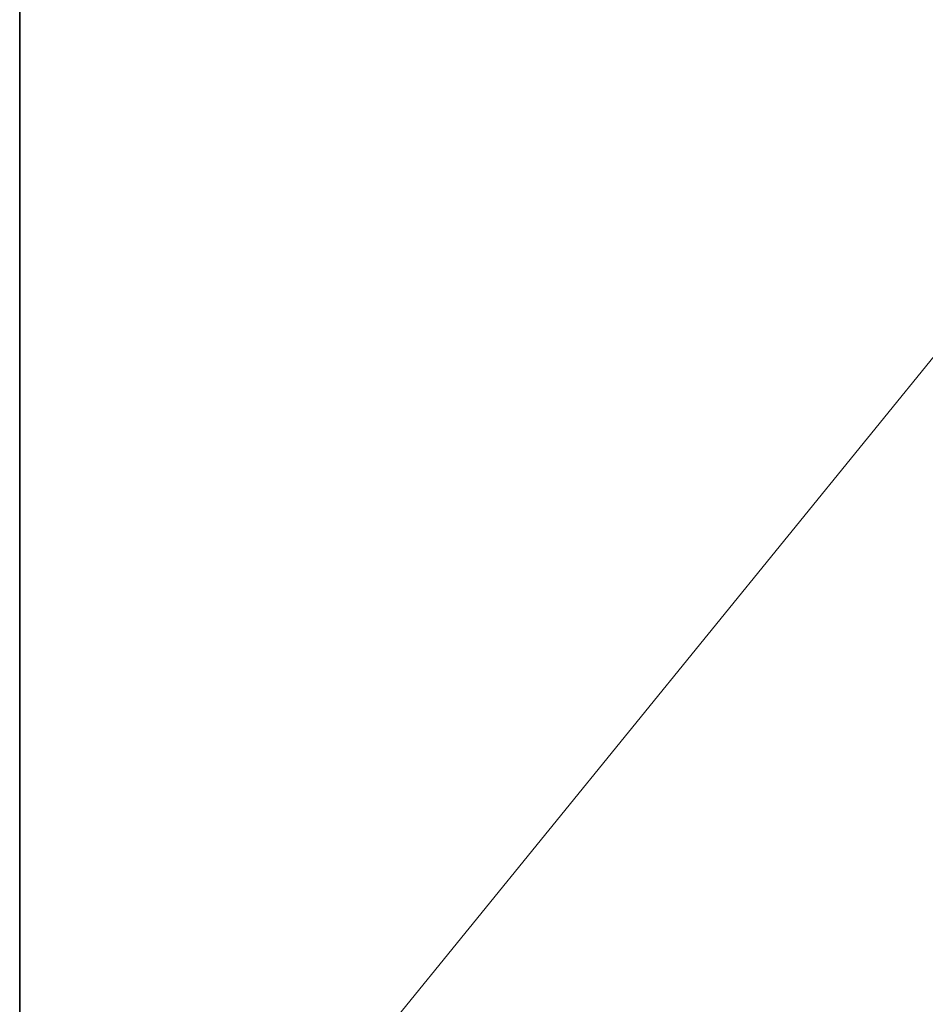
# Model space of a CAD drawing. Units: inches. Extents: x 2083 to 3317, y 1141 to 2115.
# Tile 29 of 256: x 2235.959783 to 2235.964596, y 1477.763891 to 1477.769121. Entities that reach past the tile are written whole.
import ezdxf

# ---------------------------------------------------------------- set-up
doc = ezdxf.new("R2010")
doc.units = ezdxf.units.IN
doc.linetypes.add('ACAD_ISO02W100', pattern=[15, 12, -3])
for name, color, linetype, lineweight in [('A-ANNO-DIMS', 2, 'Continuous', 18), ('A-FLOR-OPEN', 8, 'ACAD_ISO02W100', 13), ('A-WALL', 7, 'Continuous', 35)]:
    doc.layers.add(name, color=color, linetype=linetype, lineweight=lineweight)
doc.styles.get("Standard").update_dxf_attribs({"font": 'arial.ttf'})
doc.dimstyles.new('ISO-25', dxfattribs={"dimtxt": 12, "dimasz": 12, "dimexe": 1.25, "dimexo": 0.625, "dimtad": 1, "dimlunit": 3, "dimtxsty": 'Standard', "dimcen": 2.5, "dimadec": 0, "dimazin": 0, "dimtfac": 1, "dimtmove": 0, "dimatfit": 3, "dimfxl": 1, "dimarcsym": 0})

# ---------------------------------------------------------------- blocks, each defined once
blk = doc.blocks.new('*D45')
at = {"layer": 'A-ANNO-DIMS', "color": 0, "lineweight": -2, "transparency": 16777216}
for p, q in [((2235.959783, 1478.38636), (2235.959783, 1531.36136)), ((2418.959783, 1478.38636), (2418.959783, 1531.36136)), ((2247.959783, 1530.11136), (2406.959783, 1530.11136))]:
    blk.add_line(p, q, dxfattribs=at)
at = {"layer": 'A-ANNO-DIMS', "color": 0, "transparency": 16777216}
for points in [[(2247.959783, 1532.11136), (2247.959783, 1528.11136), (2235.959783, 1530.11136)], [(2406.959783, 1532.11136), (2406.959783, 1528.11136), (2418.959783, 1530.11136)]]:
    blk.add_solid(points, dxfattribs=at)
at = {"layer": 'Defpoints', "color": 0, "transparency": 16777216}
for p in [(2418.959783, 1530.11136), (2235.959783, 1477.76136), (2418.959783, 1477.76136)]:
    blk.add_point(p, dxfattribs=at)
at = {"layer": 'A-ANNO-DIMS', "color": 0, "transparency": 16777216, "insert": (2327.459783, 1536.8673286), "char_height": 12, "attachment_point": 5}
blk.add_mtext('15\'-3"', dxfattribs=at)
blk = doc.blocks.new('*D62')
at = {"layer": 'A-ANNO-DIMS', "color": 0, "lineweight": -2, "transparency": 16777216}
for p, q in [((2235.959783, 1469.38636), (2235.959783, 1522.36136)), ((2379.959783, 1469.38636), (2379.959783, 1522.36136)), ((2247.959783, 1521.11136), (2367.959783, 1521.11136))]:
    blk.add_line(p, q, dxfattribs=at)
at = {"layer": 'A-ANNO-DIMS', "color": 0, "transparency": 16777216}
for points in [[(2247.959783, 1523.11136), (2247.959783, 1519.11136), (2235.959783, 1521.11136)], [(2367.959783, 1523.11136), (2367.959783, 1519.11136), (2379.959783, 1521.11136)]]:
    blk.add_solid(points, dxfattribs=at)
at = {"layer": 'Defpoints', "color": 0, "transparency": 16777216}
for p in [(2379.959783, 1521.11136), (2235.959783, 1468.76136), (2379.959783, 1468.76136)]:
    blk.add_point(p, dxfattribs=at)
at = {"layer": 'A-ANNO-DIMS', "color": 0, "transparency": 16777216, "insert": (2307.959783, 1527.8632359), "char_height": 12, "attachment_point": 5}
blk.add_mtext('12\'-0"', dxfattribs=at)
blk = doc.blocks.new('*D64')
at = {"layer": 'A-ANNO-DIMS', "color": 0, "lineweight": -2, "transparency": 16777216}
for p, q in [((2236.584783, 1702.76136), (2289.559783, 1702.76136)), ((2288.309783, 1690.76136), (2288.309783, 1489.76136)), ((2236.584783, 1477.76136), (2289.559783, 1477.76136))]:
    blk.add_line(p, q, dxfattribs=at)
at = {"layer": 'A-ANNO-DIMS', "color": 0, "transparency": 16777216}
for points in [[(2286.309783, 1690.76136), (2290.309783, 1690.76136), (2288.309783, 1702.76136)], [(2286.309783, 1489.76136), (2290.309783, 1489.76136), (2288.309783, 1477.76136)]]:
    blk.add_solid(points, dxfattribs=at)
at = {"layer": 'Defpoints', "color": 0, "transparency": 16777216}
for p in [(2235.959783, 1702.76136), (2235.959783, 1477.76136), (2288.309783, 1477.76136)]:
    blk.add_point(p, dxfattribs=at)
at = {"layer": 'A-ANNO-DIMS', "color": 0, "transparency": 16777216, "insert": (2281.5579071, 1590.26136), "char_height": 12, "attachment_point": 5, "rotation": 90}
blk.add_mtext('18\'-9"', dxfattribs=at)

msp = doc.modelspace()

# ---------------------------------------------------------------- linework, layer by layer
at = {"layer": 'A-FLOR-OPEN'}
msp.add_line((2235.9597832, 1477.7613601), (2418.9597832, 1702.7613601), dxfattribs=at)
at = {"layer": 'A-WALL'}
msp.add_line((2235.9597832, 1702.7613601), (2235.9597832, 1477.7613601), dxfattribs=at)
msp.add_line((2235.9597832, 1702.7613601), (2235.9597832, 1477.7613601), dxfattribs=at)

# ---------------------------------------------------------------- dimensions: what is measured, and where the dimension line sits
at = {"layer": 'A-ANNO-DIMS'}
dim = msp.add_linear_dim(base=(2288.309783, 1477.76136), p1=(2235.959783, 1702.76136), p2=(2235.959783, 1477.76136), angle=270, dimstyle='ISO-25', override={"dimdec": 1, "dimlfac": 1, "dimrnd": 0, "dimzin": 1, "dimdsep": 46, "dimlunit": 4, "dimfrac": 2}, dxfattribs=at)
dim.commit()
dim.dimension.update_dxf_attribs({"geometry": '*D64', "text_midpoint": (2281.5579071, 1590.26136)})
for base, p1, p2, picture, middle in [((2418.959783, 1530.11136), (2235.959783, 1477.76136), (2418.959783, 1477.76136), '*D45', (2327.459783, 1536.8673286)), ((2379.959783, 1521.11136), (2235.959783, 1468.76136), (2379.959783, 1468.76136), '*D62', (2307.959783, 1527.8632359))]:
    dim = msp.add_linear_dim(base=base, p1=p1, p2=p2, dimstyle='ISO-25', override={"dimdec": 1, "dimlfac": 1, "dimrnd": 0, "dimzin": 1, "dimdsep": 46, "dimlunit": 4, "dimfrac": 2}, dxfattribs=at)
    dim.commit()
    dim.dimension.update_dxf_attribs({"geometry": picture, "text_midpoint": middle})

doc.saveas('drawing.dxf')
